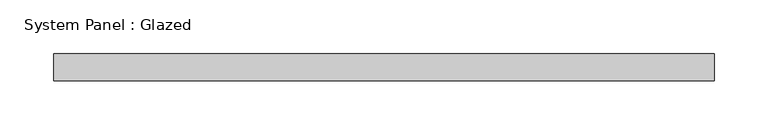
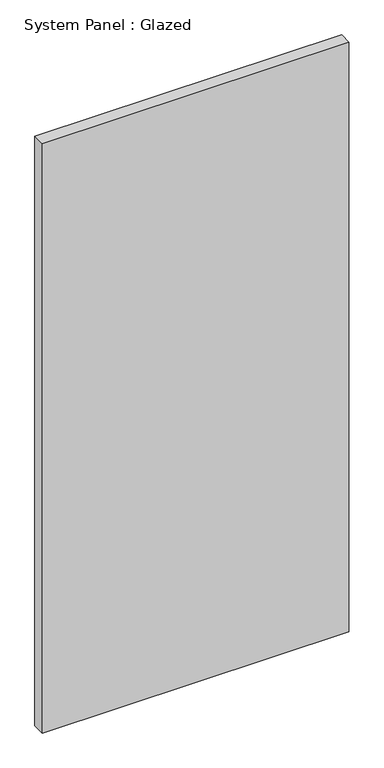
"""IFC4 building model written with IfcOpenShell, lengths in millimetres: plate geometry, System Panel : Glazed."""

from ifc_helpers import new_model, si_unit, origin, origin_with_axes, place, context, project, spatial, polyline, outline, extrude, source, transform, mapped, element, save


def system_panel_glazed_0ce4f10b(model_context):
    return source(origin(), model_context, "Body", "SweptSolid", [
        extrude(outline(polyline([(307.975, 19.05), (-307.975, 19.05), (-307.975, 44.45), (307.975, 44.45), (307.975, 19.05)])), origin_with_axes(), (0.0, 0.0, 1.0), 1251.4977008),
    ])


if __name__ == "__main__":
    model = new_model("IFC4")
    model_context = context("Model", 3, world=origin())
    ifc_project = project(units=[si_unit("LENGTHUNIT", "METRE", prefix="MILLI")], contexts=[model_context])
    site = spatial("IfcSite", under=ifc_project)
    building = spatial("IfcBuilding", under=site)
    placement = place(None, origin())
    system_panel_glazed_shape = system_panel_glazed_0ce4f10b(model_context)
    element("IfcPlate", 1, ObjectType="System Panel : Glazed", at=placement, inside=building, context=model_context, shape_type="MappedRepresentation", body=[
        mapped(system_panel_glazed_shape, transform((0.0, 0.0, 0.0), x_axis=(1.0, 0.0, 0.0), y_axis=(0.0, 1.0, 0.0), z_axis=(0.0, 0.0, 1.0))),
    ])
    save(model, "model.ifc")

# Revit data of these elements
# Type "System Panel : Glazed"
#   Construction Type Id = "GSP4R"
#   Analytic Construction = "1/8 in Pilkington single glazing"
#   Visual Light Transmittance = 0.9
#   Solar Heat Gain Coefficient = 0.86
#   Heat Transfer Coefficient (U) = 1.18115 BTU/(h·ft²·°F)
#   Define Thermal Properties by = 1
# Element 1 (IfcPlate, "System Panel : Glazed")
#   Materials on its faces: "Glass"
# Materials
#   "Glass": class "Glass", colour RGB 0 128 192, transparency 0.75, Description = "Soda Lime Glass", Cost = 0
